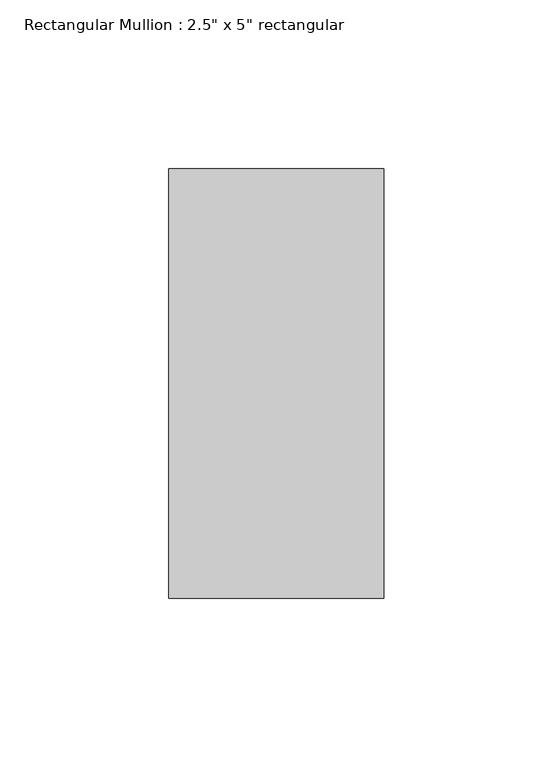
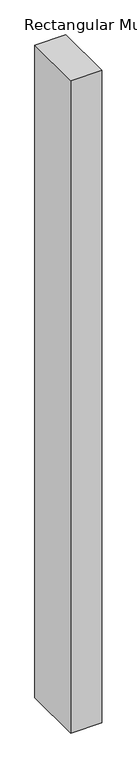
"""IFC4 building model written with IfcOpenShell, lengths in millimetres: member geometry."""

from ifc_helpers import new_model, si_unit, frame, origin, place, context, project, spatial, polyline, outline, extrude, source, transform, mapped, element, save


def member_0767621a(model_context):
    return source(origin(), model_context, "Body", "SweptSolid", [
        extrude(outline(polyline([(31.75, 63.5), (31.75, -63.5), (-31.75, -63.5), (-31.75, 63.5), (31.75, 63.5)])), frame((0.0, 0.0, -1415.2614699), z_axis=(0.0, 0.0, 1.0), x_axis=(1.0, 0.0, 0.0)), (0.0, 0.0, 1.0), 1415.2614699),
    ])


if __name__ == "__main__":
    model = new_model("IFC4")
    model_context = context("Model", 3, world=origin())
    ifc_project = project(units=[si_unit("LENGTHUNIT", "METRE", prefix="MILLI")], contexts=[model_context])
    site = spatial("IfcSite", under=ifc_project)
    building = spatial("IfcBuilding", under=site)
    placement = place(None, origin())
    member_shape = member_0767621a(model_context)
    element("IfcMember", 1, ObjectType="Rectangular Mullion : 2.5\" x 5\" rectangular", at=placement, inside=building, context=model_context, shape_type="MappedRepresentation", body=[
        mapped(member_shape, transform((0.0, 0.0, 0.0), x_axis=(1.0, 0.0, 0.0), y_axis=(0.0, 1.0, 0.0), z_axis=(0.0, 0.0, 1.0))),
    ])
    save(model, "model.ifc")

# Revit data of these elements
# Type "Rectangular Mullion : 2.5\" x 5\" rectangular"
#   built-in parameter 1007304 = 0.416667 (stored number, unit not read)
#   built-in parameter 1007301 = 0.104167 (stored number, unit not read)
#   built-in parameter 1007300 = 0.104167 (stored number, unit not read)
# Element 1 (IfcMember, "Rectangular Mullion : 2.5\" x 5\" rectangular")
#   Materials on its faces: "Aluminum"
# Materials
#   "Aluminum": class "Metal", colour RGB 247 247 247, transparency 0, Description = "Aluminum 6061", Cost = 0
